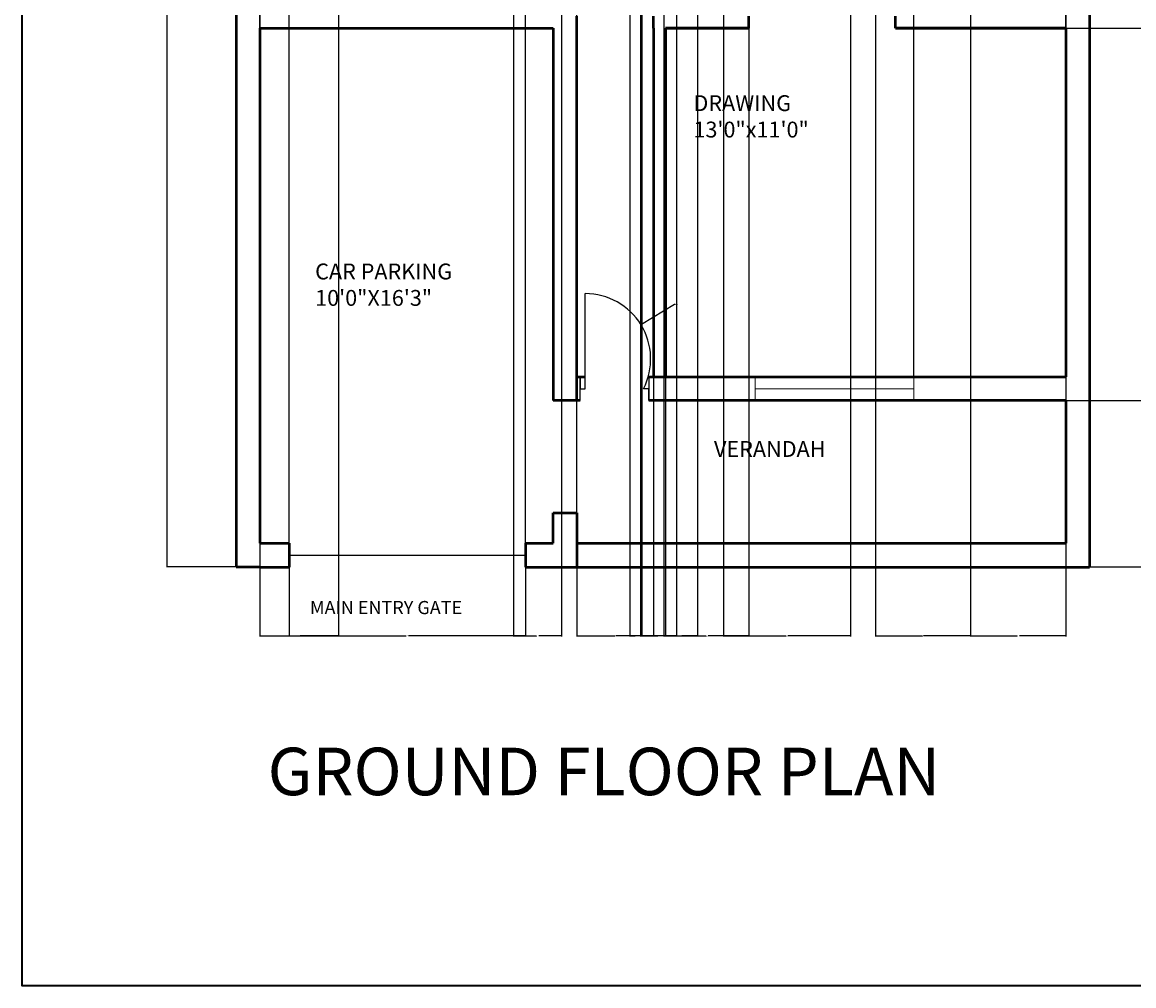
# Model space of a CAD drawing. Units: inches. Extents: x 1860 to 2753, y 1742 to 2419.
# Tile 1 of 4: x 1860 to 2280, y 1742 to 2106. Entities that reach past the tile are written whole.
import ezdxf

# ---------------------------------------------------------------- set-up
doc = ezdxf.new("R2010")
doc.units = ezdxf.units.IN
for name, color, linetype, lineweight in [('A-ANNO-DIMS', 2, 'Continuous', 18), ('A-ANNO-TEXT', 7, 'Continuous', 25), ('A-ANNO-TTLB', 7, 'Continuous', 35), ('A-AREA-IDEN', 7, 'Continuous', 18), ('A-DOOR', 3, 'Continuous', 25), ('A-GLAZ', 4, 'Continuous', 18), ('A-WALL', 7, 'Continuous', 50)]:
    doc.layers.add(name, color=color, linetype=linetype, lineweight=lineweight)
doc.styles.get("Standard").update_dxf_attribs({"font": 'arial.ttf'})
doc.dimstyles.get("Standard").update_dxf_attribs({"dimtxt": 0.18, "dimasz": 0.18, "dimexe": 0.18, "dimexo": 0.0625, "dimgap": 0.09, "dimtad": 0, "dimtih": 1, "dimtoh": 1, "dimdec": 4, "dimzin": 0, "dimdsep": 46, "dimtxsty": 'Standard', "dimcen": 0.09, "dimadec": 0, "dimazin": 0, "dimtfac": 1, "dimtdec": 4, "dimtofl": 0, "dimtmove": 0, "dimatfit": 3, "dimfxl": 1, "dimtolj": 1, "dimtzin": 0, "dimarcsym": 0})

# ---------------------------------------------------------------- blocks, each defined once
blk = doc.blocks.new('*D8')
at = {"layer": 'A-ANNO-DIMS', "color": 0, "lineweight": -2, "transparency": 16777216}
for p, q in [((1940.41, 2320.15), (1914.19, 2320.15)), ((1914.37, 2319.97), (1914.37, 2110.33)), ((1914.37, 1900.33), (1914.37, 2109.97)), ((1940.41, 1900.15), (1914.19, 1900.15))]:
    blk.add_line(p, q, dxfattribs=at)
at = {"layer": 'A-ANNO-DIMS', "color": 0, "transparency": 16777216}
for points in [[(1914.34, 2319.97), (1914.4, 2319.97), (1914.37, 2320.15)], [(1914.34, 1900.33), (1914.4, 1900.33), (1914.37, 1900.15)]]:
    blk.add_solid(points, dxfattribs=at)
at = {"layer": 'Defpoints', "color": 0, "transparency": 16777216}
for p in [(1914.37, 2320.15), (1940.47, 2320.15), (1940.47, 1900.15)]:
    blk.add_point(p, dxfattribs=at)
at = {"layer": 'A-ANNO-DIMS', "color": 0, "transparency": 16777216, "insert": (1914.37, 2110.15), "char_height": 0.18, "attachment_point": 5}
blk.add_mtext('\\A1;420', dxfattribs=at)
blk = doc.blocks.new('*D9')
at = {"layer": 'A-ANNO-DIMS', "color": 0, "lineweight": -2, "transparency": 16777216}
for p, q in [((1949.47, 2311.09), (1949.47, 1873.87)), ((1979.28, 2311.09), (1979.28, 1873.87)), ((1949.65, 1874.05), (1964, 1874.05)), ((1979.1, 1874.05), (1964.75, 1874.05))]:
    blk.add_line(p, q, dxfattribs=at)
at = {"layer": 'A-ANNO-DIMS', "color": 0, "transparency": 16777216}
for points in [[(1949.65, 1874.08), (1949.65, 1874.02), (1949.47, 1874.05)], [(1979.1, 1874.08), (1979.1, 1874.02), (1979.28, 1874.05)]]:
    blk.add_solid(points, dxfattribs=at)
at = {"layer": 'Defpoints', "color": 0, "transparency": 16777216}
for p in [(1949.47, 2311.15), (1979.28, 2311.15), (1979.28, 1874.05)]:
    blk.add_point(p, dxfattribs=at)
at = {"layer": 'A-ANNO-DIMS', "color": 0, "transparency": 16777216, "insert": (1964.37, 1874.05), "char_height": 0.18, "attachment_point": 5}
blk.add_mtext('\\A1;29.81', dxfattribs=at)
blk = doc.blocks.new('*D10')
at = {"layer": 'A-ANNO-DIMS', "color": 0, "lineweight": -2, "transparency": 16777216}
for p, q in [((2093.97, 2311.09), (2093.97, 1873.87)), ((2107.08, 2311.09), (2107.08, 1873.87)), ((2094.15, 1874.05), (2100.07, 1874.05)), ((2106.9, 1874.05), (2100.98, 1874.05))]:
    blk.add_line(p, q, dxfattribs=at)
at = {"layer": 'A-ANNO-DIMS', "color": 0, "transparency": 16777216}
for points in [[(2094.15, 1874.08), (2094.15, 1874.02), (2093.97, 1874.05)], [(2106.9, 1874.08), (2106.9, 1874.02), (2107.08, 1874.05)]]:
    blk.add_solid(points, dxfattribs=at)
at = {"layer": 'Defpoints', "color": 0, "transparency": 16777216}
for p in [(2093.97, 2311.15), (2107.08, 2311.15), (2107.08, 1874.05)]:
    blk.add_point(p, dxfattribs=at)
at = {"layer": 'A-ANNO-DIMS', "color": 0, "transparency": 16777216, "insert": (2100.52, 1874.05), "char_height": 0.18, "attachment_point": 5}
blk.add_mtext('\\A1;13.107', dxfattribs=at)
blk = doc.blocks.new('*D11')
at = {"layer": 'A-ANNO-DIMS', "color": 0, "lineweight": -2, "transparency": 16777216}
for p, q in [((2182.45, 2311.09), (2182.45, 1873.87)), ((2218.45, 2311.09), (2218.45, 1873.87)), ((2182.63, 1874.05), (2200.24, 1874.05)), ((2218.27, 1874.05), (2200.67, 1874.05))]:
    blk.add_line(p, q, dxfattribs=at)
at = {"layer": 'A-ANNO-DIMS', "color": 0, "transparency": 16777216}
for points in [[(2182.63, 1874.08), (2182.63, 1874.02), (2182.45, 1874.05)], [(2218.27, 1874.08), (2218.27, 1874.02), (2218.45, 1874.05)]]:
    blk.add_solid(points, dxfattribs=at)
at = {"layer": 'Defpoints', "color": 0, "transparency": 16777216}
for p in [(2182.45, 2311.15), (2218.45, 2311.15), (2218.45, 1874.05)]:
    blk.add_point(p, dxfattribs=at)
at = {"layer": 'A-ANNO-DIMS', "color": 0, "transparency": 16777216, "insert": (2200.45, 1874.05), "char_height": 0.18, "attachment_point": 5}
blk.add_mtext('\\A1;36', dxfattribs=at)
blk = doc.blocks.new('*D12')
at = {"layer": 'A-ANNO-DIMS', "color": 0, "lineweight": -2, "transparency": 16777216}
for p, q in [((2218.45, 2311.09), (2218.45, 1873.87)), ((2254.47, 2311.09), (2254.47, 1873.87)), ((2218.63, 1874.05), (2236, 1874.05)), ((2254.29, 1874.05), (2236.93, 1874.05))]:
    blk.add_line(p, q, dxfattribs=at)
at = {"layer": 'A-ANNO-DIMS', "color": 0, "transparency": 16777216}
for points in [[(2218.63, 1874.08), (2218.63, 1874.02), (2218.45, 1874.05)], [(2254.29, 1874.08), (2254.29, 1874.02), (2254.47, 1874.05)]]:
    blk.add_solid(points, dxfattribs=at)
at = {"layer": 'Defpoints', "color": 0, "transparency": 16777216}
for p in [(2218.45, 2311.15), (2254.47, 2311.15), (2254.47, 1874.05)]:
    blk.add_point(p, dxfattribs=at)
at = {"layer": 'A-ANNO-DIMS', "color": 0, "transparency": 16777216, "insert": (2236.46, 1874.05), "char_height": 0.18, "attachment_point": 5}
blk.add_mtext('\\A1;36.016', dxfattribs=at)
blk = doc.blocks.new('*D13')
at = {"layer": 'A-ANNO-DIMS', "color": 0, "lineweight": -2, "transparency": 16777216}
for p, q in [((1949.47, 1909.21), (1949.47, 2346.43)), ((1949.65, 2346.25), (1954.55, 2346.25)), ((1960.35, 2346.25), (1955.46, 2346.25)), ((1960.53, 1909.21), (1960.53, 2346.43))]:
    blk.add_line(p, q, dxfattribs=at)
at = {"layer": 'A-ANNO-DIMS', "color": 0, "transparency": 16777216}
for points in [[(1949.65, 2346.28), (1949.65, 2346.22), (1949.47, 2346.25)], [(1960.35, 2346.28), (1960.35, 2346.22), (1960.53, 2346.25)]]:
    blk.add_solid(points, dxfattribs=at)
at = {"layer": 'Defpoints', "color": 0, "transparency": 16777216}
for p in [(1960.53, 2346.25), (1949.47, 1909.15), (1960.53, 1909.15)]:
    blk.add_point(p, dxfattribs=at)
at = {"layer": 'A-ANNO-DIMS', "color": 0, "transparency": 16777216, "insert": (1955, 2346.25), "char_height": 0.18, "attachment_point": 5}
blk.add_mtext('\\A1;11.063', dxfattribs=at)
blk = doc.blocks.new('*D14')
at = {"layer": 'A-ANNO-DIMS', "color": 0, "lineweight": -2, "transparency": 16777216}
for p, q in [((1960.53, 1900.09), (1960.53, 1873.87)), ((2050.02, 1900.09), (2050.02, 1873.87)), ((1960.71, 1874.05), (2004.88, 1874.05)), ((2049.84, 1874.05), (2005.67, 1874.05))]:
    blk.add_line(p, q, dxfattribs=at)
at = {"layer": 'A-ANNO-DIMS', "color": 0, "transparency": 16777216}
for points in [[(1960.71, 1874.08), (1960.71, 1874.02), (1960.53, 1874.05)], [(2049.84, 1874.08), (2049.84, 1874.02), (2050.02, 1874.05)]]:
    blk.add_solid(points, dxfattribs=at)
at = {"layer": 'Defpoints', "color": 0, "transparency": 16777216}
for p in [(1960.53, 1900.15), (2050.02, 1900.15), (2050.02, 1874.05)]:
    blk.add_point(p, dxfattribs=at)
at = {"layer": 'A-ANNO-DIMS', "color": 0, "transparency": 16777216, "insert": (2005.28, 1874.05), "char_height": 0.18, "attachment_point": 5}
blk.add_mtext('\\A1;89.49', dxfattribs=at)
blk = doc.blocks.new('*D15')
at = {"layer": 'A-ANNO-DIMS', "color": 0, "lineweight": -2, "transparency": 16777216}
for p, q in [((2050.02, 1909.21), (2050.02, 2346.43)), ((2050.2, 2346.25), (2059.36, 2346.25)), ((2069.29, 2346.25), (2060.13, 2346.25)), ((2069.47, 1920.76), (2069.47, 2346.43))]:
    blk.add_line(p, q, dxfattribs=at)
at = {"layer": 'A-ANNO-DIMS', "color": 0, "transparency": 16777216}
for points in [[(2050.2, 2346.28), (2050.2, 2346.22), (2050.02, 2346.25)], [(2069.29, 2346.28), (2069.29, 2346.22), (2069.47, 2346.25)]]:
    blk.add_solid(points, dxfattribs=at)
at = {"layer": 'Defpoints', "color": 0, "transparency": 16777216}
for p in [(2069.47, 2346.25), (2069.47, 1920.7), (2050.02, 1909.15)]:
    blk.add_point(p, dxfattribs=at)
at = {"layer": 'A-ANNO-DIMS', "color": 0, "transparency": 16777216, "insert": (2059.74, 2346.25), "char_height": 0.18, "attachment_point": 5}
blk.add_mtext('\\A1;19.45', dxfattribs=at)
blk = doc.blocks.new('*D16')
at = {"layer": 'A-ANNO-DIMS', "color": 0, "lineweight": -2, "transparency": 16777216}
for p, q in [((2098.47, 1972.09), (2098.47, 1873.87)), ((2069.47, 1900.09), (2069.47, 1873.87)), ((2069.65, 1874.05), (2083.75, 1874.05)), ((2098.29, 1874.05), (2084.19, 1874.05))]:
    blk.add_line(p, q, dxfattribs=at)
at = {"layer": 'A-ANNO-DIMS', "color": 0, "transparency": 16777216}
for points in [[(2069.65, 1874.08), (2069.65, 1874.02), (2069.47, 1874.05)], [(2098.29, 1874.08), (2098.29, 1874.02), (2098.47, 1874.05)]]:
    blk.add_solid(points, dxfattribs=at)
at = {"layer": 'Defpoints', "color": 0, "transparency": 16777216}
for p in [(2098.47, 1972.15), (2069.47, 1900.15), (2098.47, 1874.05)]:
    blk.add_point(p, dxfattribs=at)
at = {"layer": 'A-ANNO-DIMS', "color": 0, "transparency": 16777216, "insert": (2083.97, 1874.05), "char_height": 0.18, "attachment_point": 5}
blk.add_mtext('\\A1;29', dxfattribs=at)
blk = doc.blocks.new('*D17')
at = {"layer": 'A-ANNO-DIMS', "color": 0, "lineweight": -2, "transparency": 16777216}
for p, q in [((2254.53, 1963.15), (2289.75, 1963.15)), ((2289.57, 1962.97), (2289.57, 1931.83)), ((2289.57, 1900.33), (2289.57, 1931.47)), ((2263.53, 1900.15), (2289.75, 1900.15))]:
    blk.add_line(p, q, dxfattribs=at)
at = {"layer": 'A-ANNO-DIMS', "color": 0, "transparency": 16777216}
for points in [[(2289.54, 1962.97), (2289.6, 1962.97), (2289.57, 1963.15)], [(2289.54, 1900.33), (2289.6, 1900.33), (2289.57, 1900.15)]]:
    blk.add_solid(points, dxfattribs=at)
at = {"layer": 'Defpoints', "color": 0, "transparency": 16777216}
for p in [(2254.47, 1963.15), (2289.57, 1963.15), (2263.47, 1900.15)]:
    blk.add_point(p, dxfattribs=at)
at = {"layer": 'A-ANNO-DIMS', "color": 0, "transparency": 16777216, "insert": (2289.57, 1931.65), "char_height": 0.18, "attachment_point": 5}
blk.add_mtext('\\A1;63', dxfattribs=at)
blk = doc.blocks.new('*D18')
at = {"layer": 'A-ANNO-DIMS', "color": 0, "lineweight": -2, "transparency": 16777216}
for p, q in [((2254.53, 2104.15), (2289.75, 2104.15)), ((2289.57, 2103.97), (2289.57, 2033.83)), ((2289.57, 1963.33), (2289.57, 2033.47)), ((2254.53, 1963.15), (2289.75, 1963.15))]:
    blk.add_line(p, q, dxfattribs=at)
at = {"layer": 'A-ANNO-DIMS', "color": 0, "transparency": 16777216}
for points in [[(2289.54, 2103.97), (2289.6, 2103.97), (2289.57, 2104.15)], [(2289.54, 1963.33), (2289.6, 1963.33), (2289.57, 1963.15)]]:
    blk.add_solid(points, dxfattribs=at)
at = {"layer": 'Defpoints', "color": 0, "transparency": 16777216}
for p in [(2254.47, 2104.15), (2289.57, 2104.15), (2254.47, 1963.15)]:
    blk.add_point(p, dxfattribs=at)
at = {"layer": 'A-ANNO-DIMS', "color": 0, "transparency": 16777216, "insert": (2289.57, 2033.65), "char_height": 0.18, "attachment_point": 5}
blk.add_mtext('\\A1;141', dxfattribs=at)
blk = doc.blocks.new('*D19')
at = {"layer": 'A-ANNO-DIMS', "color": 0, "lineweight": -2, "transparency": 16777216}
for p, q in [((2263.53, 2122.97), (2289.75, 2122.97)), ((2289.57, 2122.79), (2289.57, 2113.74)), ((2289.57, 2104.33), (2289.57, 2113.38)), ((2254.53, 2104.15), (2289.75, 2104.15))]:
    blk.add_line(p, q, dxfattribs=at)
at = {"layer": 'A-ANNO-DIMS', "color": 0, "transparency": 16777216}
for points in [[(2289.54, 2122.79), (2289.6, 2122.79), (2289.57, 2122.97)], [(2289.54, 2104.33), (2289.6, 2104.33), (2289.57, 2104.15)]]:
    blk.add_solid(points, dxfattribs=at)
at = {"layer": 'Defpoints', "color": 0, "transparency": 16777216}
for p in [(2263.47, 2122.97), (2289.57, 2122.97), (2254.47, 2104.15)]:
    blk.add_point(p, dxfattribs=at)
at = {"layer": 'A-ANNO-DIMS', "color": 0, "transparency": 16777216, "insert": (2289.57, 2113.56), "char_height": 0.18, "attachment_point": 5}
blk.add_mtext('\\A1;18.82', dxfattribs=at)
blk = doc.blocks.new('*D22')
at = {"layer": 'A-ANNO-DIMS', "color": 0, "lineweight": -2, "transparency": 16777216}
for p, q in [((2196.96, 1972.21), (2196.96, 2346.43)), ((2197.14, 2346.25), (2225.34, 2346.25)), ((2254.29, 2346.25), (2226.09, 2346.25)), ((2254.47, 1972.21), (2254.47, 2346.43))]:
    blk.add_line(p, q, dxfattribs=at)
at = {"layer": 'A-ANNO-DIMS', "color": 0, "transparency": 16777216}
for points in [[(2197.14, 2346.28), (2197.14, 2346.22), (2196.96, 2346.25)], [(2254.29, 2346.28), (2254.29, 2346.22), (2254.47, 2346.25)]]:
    blk.add_solid(points, dxfattribs=at)
at = {"layer": 'Defpoints', "color": 0, "transparency": 16777216}
for p in [(2254.47, 2346.25), (2196.96, 1972.15), (2254.47, 1972.15)]:
    blk.add_point(p, dxfattribs=at)
at = {"layer": 'A-ANNO-DIMS', "color": 0, "transparency": 16777216, "insert": (2225.71, 2346.25), "char_height": 0.18, "attachment_point": 5}
blk.add_mtext('\\A1;57.51', dxfattribs=at)
blk = doc.blocks.new('*D23')
at = {"layer": 'A-ANNO-DIMS', "color": 0, "lineweight": -2, "transparency": 16777216}
for p, q in [((2102.97, 2104.09), (2102.97, 1873.87)), ((2134.51, 2104.09), (2134.51, 1873.87)), ((2103.15, 1874.05), (2118.35, 1874.05)), ((2134.33, 1874.05), (2119.14, 1874.05))]:
    blk.add_line(p, q, dxfattribs=at)
at = {"layer": 'A-ANNO-DIMS', "color": 0, "transparency": 16777216}
for points in [[(2103.15, 1874.08), (2103.15, 1874.02), (2102.97, 1874.05)], [(2134.33, 1874.08), (2134.33, 1874.02), (2134.51, 1874.05)]]:
    blk.add_solid(points, dxfattribs=at)
at = {"layer": 'Defpoints', "color": 0, "transparency": 16777216}
for p in [(2102.97, 2104.15), (2134.51, 2104.15), (2134.51, 1874.05)]:
    blk.add_point(p, dxfattribs=at)
at = {"layer": 'A-ANNO-DIMS', "color": 0, "transparency": 16777216, "insert": (2118.74, 1874.05), "char_height": 0.18, "attachment_point": 5}
blk.add_mtext('\\A1;31.54', dxfattribs=at)
blk = doc.blocks.new('*D25')
at = {"layer": 'A-ANNO-DIMS', "color": 0, "lineweight": -2, "transparency": 16777216}
for p, q in [((2124.88, 2186.59), (2124.88, 1873.87)), ((2172.98, 2186.59), (2172.98, 1873.87)), ((2125.06, 1874.05), (2148.62, 1874.05)), ((2172.8, 1874.05), (2149.24, 1874.05))]:
    blk.add_line(p, q, dxfattribs=at)
at = {"layer": 'A-ANNO-DIMS', "color": 0, "transparency": 16777216}
for points in [[(2125.06, 1874.08), (2125.06, 1874.02), (2124.88, 1874.05)], [(2172.8, 1874.08), (2172.8, 1874.02), (2172.98, 1874.05)]]:
    blk.add_solid(points, dxfattribs=at)
at = {"layer": 'Defpoints', "color": 0, "transparency": 16777216}
for p in [(2124.88, 2186.65), (2172.98, 2186.65), (2172.98, 1874.05)]:
    blk.add_point(p, dxfattribs=at)
at = {"layer": 'A-ANNO-DIMS', "color": 0, "transparency": 16777216, "insert": (2148.93, 1874.05), "char_height": 0.18, "attachment_point": 5}
blk.add_mtext('\\A1;48.1', dxfattribs=at)
blk = doc.blocks.new('*D27')
at = {"layer": 'A-ANNO-DIMS', "color": 0, "lineweight": -2, "transparency": 16777216}
for p, q in [((2089.47, 2311.09), (2089.47, 1873.87)), ((2093.97, 2311.09), (2093.97, 1873.87)), ((2089.65, 1874.05), (2091.46, 1874.05)), ((2093.79, 1874.05), (2091.98, 1874.05))]:
    blk.add_line(p, q, dxfattribs=at)
at = {"layer": 'A-ANNO-DIMS', "color": 0, "transparency": 16777216}
for points in [[(2089.65, 1874.08), (2089.65, 1874.02), (2089.47, 1874.05)], [(2093.79, 1874.08), (2093.79, 1874.02), (2093.97, 1874.05)]]:
    blk.add_solid(points, dxfattribs=at)
at = {"layer": 'Defpoints', "color": 0, "transparency": 16777216}
for p in [(2089.47, 2311.15), (2093.97, 2311.15), (2093.97, 1874.05)]:
    blk.add_point(p, dxfattribs=at)
at = {"layer": 'A-ANNO-DIMS', "color": 0, "transparency": 16777216, "insert": (2091.72, 1874.05), "char_height": 0.18, "attachment_point": 5}
blk.add_mtext('\\A1;4.5', dxfattribs=at)
blk = doc.blocks.new('*D28')
at = {"layer": 'A-ANNO-DIMS', "color": 0, "lineweight": -2, "transparency": 16777216}
for p, q in [((2102.3, 2222.59), (2102.3, 1873.87)), ((2115.14, 2222.59), (2115.14, 1873.87)), ((2102.48, 1874.05), (2108.27, 1874.05)), ((2114.96, 1874.05), (2109.18, 1874.05))]:
    blk.add_line(p, q, dxfattribs=at)
at = {"layer": 'A-ANNO-DIMS', "color": 0, "transparency": 16777216}
for points in [[(2102.48, 1874.08), (2102.48, 1874.02), (2102.3, 1874.05)], [(2114.96, 1874.08), (2114.96, 1874.02), (2115.14, 1874.05)]]:
    blk.add_solid(points, dxfattribs=at)
at = {"layer": 'Defpoints', "color": 0, "transparency": 16777216}
for p in [(2102.3, 2222.65), (2115.14, 2222.65), (2115.14, 1874.05)]:
    blk.add_point(p, dxfattribs=at)
at = {"layer": 'A-ANNO-DIMS', "color": 0, "transparency": 16777216, "insert": (2108.72, 1874.05), "char_height": 0.18, "attachment_point": 5}
blk.add_mtext('\\A1;12.834', dxfattribs=at)
blk = doc.blocks.new('*D29')
at = {"layer": 'A-ANNO-DIMS', "color": 0, "lineweight": -2, "transparency": 16777216}
for p, q in [((2102.3, 2191.09), (2102.3, 1873.87)), ((2093.49, 2186.59), (2093.49, 1873.87)), ((2093.67, 1874.05), (2097.51, 1874.05)), ((2102.12, 1874.05), (2098.29, 1874.05))]:
    blk.add_line(p, q, dxfattribs=at)
at = {"layer": 'A-ANNO-DIMS', "color": 0, "transparency": 16777216}
for points in [[(2093.67, 1874.08), (2093.67, 1874.02), (2093.49, 1874.05)], [(2102.12, 1874.08), (2102.12, 1874.02), (2102.3, 1874.05)]]:
    blk.add_solid(points, dxfattribs=at)
at = {"layer": 'Defpoints', "color": 0, "transparency": 16777216}
for p in [(2102.3, 2191.15), (2093.49, 2186.65), (2102.3, 1874.05)]:
    blk.add_point(p, dxfattribs=at)
at = {"layer": 'A-ANNO-DIMS', "color": 0, "transparency": 16777216, "insert": (2097.9, 1874.05), "char_height": 0.18, "attachment_point": 5}
blk.add_mtext('\\A1;8.809', dxfattribs=at)
blk = doc.blocks.new('*D30')
at = {"layer": 'A-ANNO-DIMS', "color": 0, "lineweight": -2, "transparency": 16777216}
for p, q in [((2045.47, 2186.59), (2045.47, 1873.87)), ((2063.65, 2186.59), (2063.65, 1873.87)), ((2045.65, 1874.05), (2054.11, 1874.05)), ((2063.47, 1874.05), (2055.02, 1874.05))]:
    blk.add_line(p, q, dxfattribs=at)
at = {"layer": 'A-ANNO-DIMS', "color": 0, "transparency": 16777216}
for points in [[(2045.65, 1874.08), (2045.65, 1874.02), (2045.47, 1874.05)], [(2063.47, 1874.08), (2063.47, 1874.02), (2063.65, 1874.05)]]:
    blk.add_solid(points, dxfattribs=at)
at = {"layer": 'Defpoints', "color": 0, "transparency": 16777216}
for p in [(2045.47, 2186.65), (2063.65, 2186.65), (2063.65, 1874.05)]:
    blk.add_point(p, dxfattribs=at)
at = {"layer": 'A-ANNO-DIMS', "color": 0, "transparency": 16777216, "insert": (2054.56, 1874.05), "char_height": 0.18, "attachment_point": 5}
blk.add_mtext('\\A1;18.183', dxfattribs=at)
blk = doc.blocks.new('*D54')
at = {"layer": 'A-ANNO-DIMS', "color": 0, "lineweight": -2, "transparency": 16777216}
for p, q in [((2106.4, 1999.58), (2093.89, 1991.92)), ((2106.58, 1999.58), (2106.4, 1999.58)), ((2072.54, 1978.9), (2072.72, 1978.9)), ((2072.63, 1978.81), (2072.63, 1978.99))]:
    blk.add_line(p, q, dxfattribs=at)
at = {"layer": 'A-ANNO-DIMS', "color": 0, "transparency": 16777216}
blk.add_solid([(2093.87, 1991.94), (2093.9, 1991.89), (2093.73, 1991.82)], dxfattribs=at)
at = {"layer": 'Defpoints', "color": 0, "transparency": 16777216}
for p in [(2093.73, 1991.82), (2072.63, 1978.9)]:
    blk.add_point(p, dxfattribs=at)
at = {"layer": 'A-ANNO-DIMS', "color": 0, "transparency": 16777216, "insert": (2107.13, 1999.58), "char_height": 0.18, "attachment_point": 5}
blk.add_mtext('\\A1;R24.747', dxfattribs=at)

msp = doc.modelspace()

# ---------------------------------------------------------------- linework, layer by layer
at = {"layer": 'A-ANNO-TTLB'}
msp.add_lwpolyline([(1859.5561, 2419.29), (2753.3204, 2419.29), (2753.3204, 1741.6035), (1859.5561, 1741.6035)], close=True, dxfattribs=at)
at = {"layer": 'A-DOOR'}
for p, q in [((2072.6268, 1967.6476), (2072.6268, 2003.6476)), ((2070.6268, 1963.1476), (2070.6268, 1972.1476)), ((2070.6268, 1972.1476), (2070.6268, 1967.6476)), ((2096.6673, 1972.1476), (2096.6673, 1972.1476)), ((2096.6673, 1972.1476), (2096.6673, 1963.1476)), ((2070.6268, 1967.6476), (2072.6268, 1967.6476)), ((2096.6673, 1967.6476), (2094.6673, 1967.6476)), ((2096.6673, 1963.1476), (2096.6673, 1967.6476)), ((1960.5331, 1904.6476), (2050.0189, 1904.6476))]:
    msp.add_line(p, q, dxfattribs=at)
msp.add_arc((2072.6268, 1978.9006), 24.747, 332.952921, 90, dxfattribs=at)
at = {"layer": 'A-GLAZ'}
for p, q in [((2136.9581, 1972.1476), (2136.9581, 1963.1476)), ((2196.9581, 1967.6476), (2196.9581, 1972.1476)), ((2196.9581, 1972.1476), (2196.9581, 1963.1476)), ((2136.9581, 1963.1476), (2136.9581, 1967.6476)), ((2136.9581, 1967.6476), (2184.9581, 1967.6476)), ((2184.9581, 1967.6476), (2196.9581, 1967.6476))]:
    msp.add_line(p, q, dxfattribs=at)
at = {"layer": 'A-WALL'}
for p, q in [((1940.4703, 2320.1476), (1940.4703, 1900.1476)), ((2263.4703, 2320.1476), (2263.4703, 1900.1476)), ((2069.4703, 1963.1476), (2069.4703, 2108.6476)), ((2098.4703, 2104.1476), (2098.4703, 2108.6476)), ((2134.5133, 2104.1476), (2134.5133, 2108.6476)), ((2189.9627, 2104.1476), (2189.9627, 2108.6476)), ((1949.4703, 2104.1476), (2060.4703, 2104.1476)), ((1949.4703, 2104.1476), (1949.4703, 1909.1476)), ((2060.4703, 2104.1476), (2060.4703, 1963.1476)), ((2098.4703, 2104.1476), (2098.4703, 1972.1476)), ((2102.9703, 2104.1476), (2134.5133, 2104.1476)), ((2134.5133, 2104.1476), (2102.9703, 2104.1476)), ((2102.9703, 2104.1476), (2102.9703, 1972.1476)), ((2102.9703, 1972.1476), (2102.9703, 2104.1476)), ((2254.4703, 2104.1476), (2189.9627, 2104.1476)), ((2189.9627, 2104.1476), (2254.4703, 2104.1476)), ((2254.4703, 2104.1476), (2254.4703, 1972.1476)), ((2069.4703, 1963.1476), (2069.4703, 1972.1476)), ((2069.4703, 1972.1476), (2072.6268, 1972.1476)), ((2096.4346, 1972.1476), (2098.4703, 1972.1476)), ((2098.4703, 1972.1476), (2102.9703, 1972.1476)), ((2102.9703, 1972.1476), (2254.4703, 1972.1476)), ((2102.9703, 1972.1476), (2102.9703, 1972.1476)), ((2070.6268, 1963.1476), (2060.4703, 1963.1476)), ((2254.4703, 1963.1476), (2096.6673, 1963.1476)), ((2254.4703, 1963.1476), (2254.4703, 1909.1476)), ((2060.4703, 1909.1476), (2060.4703, 1920.6989)), ((2060.4703, 1920.6989), (2069.4703, 1920.6989)), ((2069.4703, 1920.6989), (2069.4703, 1900.1476)), ((1949.4703, 1909.1476), (1960.5331, 1909.1476)), ((1949.4703, 1909.1476), (1960.5331, 1909.1476)), ((1960.5331, 1909.1476), (1960.5331, 1900.1476)), ((2050.0189, 1909.1476), (2050.0189, 1900.1476)), ((2050.0189, 1909.1476), (2060.4703, 1909.1476)), ((2050.0189, 1909.1476), (2060.4703, 1909.1476)), ((2069.4703, 1909.1476), (2254.4703, 1909.1476)), ((2098.4703, 1909.1476), (2102.9703, 1909.1476)), ((1949.4703, 1900.1476), (1940.4703, 1900.1476)), ((1949.4703, 1900.1476), (1960.5331, 1900.1476)), ((1949.4703, 1900.1476), (1960.5331, 1900.1476)), ((2050.0189, 1900.1476), (2069.4703, 1900.1476)), ((2050.0189, 1900.1476), (2263.4703, 1900.1476))]:
    msp.add_line(p, q, dxfattribs=at)

# ---------------------------------------------------------------- texts
at = {"layer": 'A-ANNO-TEXT', "attachment_point": 1}
for s, width, insert, char_height in [('MAIN ENTRY GATE', 126.344311, (1968.4215, 1887.2929), 5), ('GROUND FLOOR PLAN ', 369.132173, (1952.4161, 1831.7475), 18)]:
    msp.add_mtext_dynamic_manual_height_columns(s, width=width, gutter_width=12.5, heights=[0], dxfattribs=dict(at, insert=insert, char_height=char_height))
at = {"layer": 'A-AREA-IDEN', "char_height": 6, "attachment_point": 1}
for s, width, insert in [('DRAWING\\P13\'0"x11\'0"', 272.910464, (2113.5556, 2078.762)), ('CAR PARKING\\P10\'0"X16\'3"', 269.913844, (1970.4029, 2015.0308)), ('VERANDAH', 175.454231, (2121.3281, 1947.8329))]:
    msp.add_mtext_dynamic_manual_height_columns(s, width=width, gutter_width=12.5, heights=[0], dxfattribs=dict(at, insert=insert))

# ---------------------------------------------------------------- dimensions: what is measured, and where the dimension line sits
at = {"layer": 'A-ANNO-DIMS'}
for base, p1, p2, override, picture, middle in [((1960.5331, 2346.2476), (1949.4703, 1909.1476), (1960.5331, 1909.1476), {"dimdec": 3, "dimlfac": 1, "dimrnd": 0, "dimzin": 0, "dimdsep": 46, "dimlunit": 2}, '*D13', (1955.0017, 2346.2476)), ((2069.4703, 2346.2476), (2050.0189, 1909.1476), (2069.4703, 1920.6989), {"dimdec": 2, "dimlfac": 1, "dimrnd": 0, "dimzin": 0, "dimdsep": 46, "dimlunit": 2}, '*D15', (2059.7446, 2346.2476)), ((2254.4703, 2346.2476), (2196.9581, 1972.1476), (2254.4703, 1972.1476), {"dimdec": 2, "dimlfac": 1, "dimrnd": 0, "dimzin": 0, "dimdsep": 46, "dimlunit": 2}, '*D22', (2225.7142, 2346.2476)), ((1979.2792, 1874.0476), (1949.4703, 2311.1476), (1979.2792, 2311.1476), {"dimdec": 2, "dimlfac": 1, "dimrnd": 0, "dimzin": 0, "dimdsep": 46, "dimlunit": 2}, '*D9', (1964.3747, 1874.0476)), ((2093.9703, 1874.0476), (2089.4703, 2311.1476), (2093.9703, 2311.1476), {"dimdec": 1, "dimlfac": 1, "dimrnd": 0, "dimzin": 0, "dimdsep": 46, "dimlunit": 2}, '*D27', (2091.7203, 1874.0476)), ((2107.0777, 1874.0476), (2093.9703, 2311.1476), (2107.0777, 2311.1476), {"dimdec": 3, "dimlfac": 1, "dimrnd": 0, "dimzin": 0, "dimdsep": 46, "dimlunit": 2}, '*D10', (2100.524, 1874.0476)), ((2218.4546, 1874.0476), (2182.4546, 2311.1476), (2218.4546, 2311.1476), {"dimdec": 0, "dimlfac": 1, "dimrnd": 0, "dimzin": 0, "dimdsep": 46, "dimlunit": 2}, '*D11', (2200.4546, 1874.0476)), ((2254.4703, 1874.0476), (2218.4546, 2311.1476), (2254.4703, 2311.1476), {"dimdec": 3, "dimlfac": 1, "dimrnd": 0, "dimzin": 0, "dimdsep": 46, "dimlunit": 2}, '*D12', (2236.4625, 1874.0476)), ((2115.1377, 1874.0476), (2102.304, 2222.6476), (2115.1377, 2222.6476), {"dimdec": 3, "dimlfac": 1, "dimrnd": 0, "dimzin": 0, "dimdsep": 46, "dimlunit": 2}, '*D28', (2108.7208, 1874.0476)), ((2102.304, 1874.0476), (2093.4949, 2186.6476), (2102.304, 2191.1476), {"dimdec": 3, "dimlfac": 1, "dimrnd": 0, "dimzin": 0, "dimdsep": 46, "dimlunit": 2}, '*D29', (2097.8994, 1874.0476)), ((2063.6532, 1874.0476), (2045.4703, 2186.6476), (2063.6532, 2186.6476), {"dimdec": 3, "dimlfac": 1, "dimrnd": 0, "dimzin": 0, "dimdsep": 46, "dimlunit": 2}, '*D30', (2054.5618, 1874.0476)), ((2172.9826, 1874.0476), (2124.8791, 2186.6476), (2172.9826, 2186.6476), {"dimdec": 1, "dimlfac": 1, "dimrnd": 0, "dimzin": 0, "dimdsep": 46, "dimlunit": 2}, '*D25', (2148.9308, 1874.0476)), ((2134.5133, 1874.0476), (2102.9703, 2104.1476), (2134.5133, 2104.1476), {"dimdec": 2, "dimlfac": 1, "dimrnd": 0, "dimzin": 0, "dimdsep": 46, "dimlunit": 2}, '*D23', (2118.7418, 1874.0476)), ((2098.4703, 1874.0476), (2069.4703, 1900.1476), (2098.4703, 1972.1476), {"dimdec": 0, "dimlfac": 1, "dimrnd": 0, "dimzin": 0, "dimdsep": 46, "dimlunit": 2}, '*D16', (2083.9703, 1874.0476)), ((2050.0189, 1874.0476), (1960.5331, 1900.1476), (2050.0189, 1900.1476), {"dimdec": 2, "dimlfac": 1, "dimrnd": 0, "dimzin": 0, "dimdsep": 46, "dimlunit": 2}, '*D14', (2005.276, 1874.0476))]:
    dim = msp.add_linear_dim(base=base, p1=p1, p2=p2, dimstyle='Standard', override=override, dxfattribs=at)
    dim.commit()
    dim.dimension.update_dxf_attribs({"geometry": picture, "text_midpoint": middle})
for base, p1, p2, override, picture, middle in [((1914.3703, 2320.1476), (1940.4703, 1900.1476), (1940.4703, 2320.1476), {"dimdec": 0, "dimlfac": 1, "dimrnd": 0, "dimzin": 0, "dimdsep": 46, "dimlunit": 2}, '*D8', (1914.3703, 2110.1476)), ((2289.5703, 2122.9674), (2254.4703, 2104.1476), (2263.4703, 2122.9674), {"dimdec": 2, "dimlfac": 1, "dimrnd": 0, "dimzin": 0, "dimdsep": 46, "dimlunit": 2}, '*D19', (2289.5703, 2113.5575)), ((2289.5703, 2104.1476), (2254.4703, 1963.1476), (2254.4703, 2104.1476), {"dimdec": 0, "dimlfac": 1, "dimrnd": 0, "dimzin": 0, "dimdsep": 46, "dimlunit": 2}, '*D18', (2289.5703, 2033.6476)), ((2289.5703, 1963.1476), (2263.4703, 1900.1476), (2254.4703, 1963.1476), {"dimdec": 0, "dimlfac": 1, "dimrnd": 0, "dimzin": 0, "dimdsep": 46, "dimlunit": 2}, '*D17', (2289.5703, 1931.6476))]:
    dim = msp.add_linear_dim(base=base, p1=p1, p2=p2, angle=90, dimstyle='Standard', override=override, dxfattribs=at)
    dim.commit()
    dim.dimension.update_dxf_attribs({"geometry": picture, "text_midpoint": middle})
dim = msp.add_radius_dim(center=(2072.6268, 1978.9006), mpoint=(2093.7324, 1991.8222), dimstyle='Standard', override={"dimdec": 3, "dimlfac": 1, "dimrnd": 0, "dimzin": 0, "dimdsep": 46, "dimlunit": 2}, dxfattribs=at)
dim.commit()
dim.dimension.update_dxf_attribs({"geometry": '*D54', "text_midpoint": (2107.1255, 1999.5752), "dimtype": 164})

doc.saveas('drawing.dxf')
